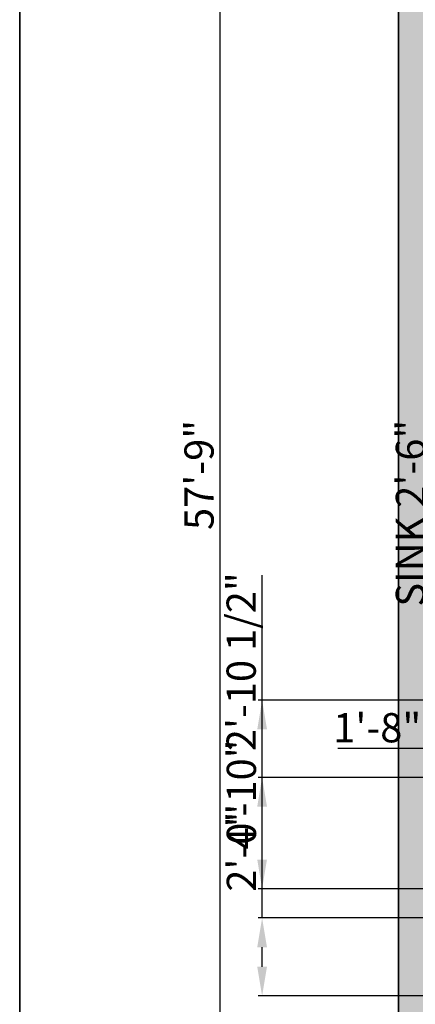
# Model space of a CAD drawing. Units: inches. Extents: x 32476 to 33108, y 58720 to 59630.
# Tile 2 of 6: x 32476 to 32598, y 58975 to 59278. Entities that reach past the tile are written whole.
import ezdxf

# ---------------------------------------------------------------- set-up
doc = ezdxf.new("R2010")
doc.units = ezdxf.units.IN
for name, color, linetype, lineweight in [('A-ANNO-DIMS', 6, 'Continuous', 18), ('A-ANNO-TTLB', 7, 'Continuous', 35), ('A-WALL', 7, 'Continuous', 35), ('A-WALL-PATT', 251, 'Continuous', 13)]:
    doc.layers.add(name, color=color, linetype=linetype, lineweight=lineweight)
doc.styles.get("Standard").update_dxf_attribs({"font": 'arial.ttf'})
doc.dimstyles.new('ISO-25', dxfattribs={"dimtxt": 9, "dimasz": 9, "dimexe": 1.25, "dimexo": 0.625, "dimtad": 1, "dimdec": 1, "dimrnd": 9, "dimlunit": 3, "dimtxsty": 'Standard', "dimcen": 2.5, "dimadec": 0, "dimazin": 0, "dimtfac": 1, "dimtdec": 1, "dimtmove": 0, "dimatfit": 3, "dimfxl": 1, "dimarcsym": 0})

# ---------------------------------------------------------------- blocks, each defined once
blk = doc.blocks.new('*D2')
at = {"layer": 'A-ANNO-DIMS', "color": 0, "lineweight": -2, "transparency": 16777216}
for p, q in [((32592.41, 59486.22), (32536.75, 59486.22)), ((32538, 59477.22), (32538, 58799.22)), ((32592.41, 58790.22), (32536.75, 58790.22))]:
    blk.add_line(p, q, dxfattribs=at)
at = {"layer": 'A-ANNO-DIMS', "color": 0, "transparency": 16777216}
for points in [[(32536.5, 59477.22), (32539.5, 59477.22), (32538, 59486.22)], [(32536.5, 58799.22), (32539.5, 58799.22), (32538, 58790.22)]]:
    blk.add_solid(points, dxfattribs=at)
at = {"layer": 'Defpoints', "color": 0, "transparency": 16777216}
for p in [(32593.04, 59486.22), (32538, 58790.22), (32593.04, 58790.22)]:
    blk.add_point(p, dxfattribs=at)
at = {"layer": 'A-ANNO-DIMS', "color": 0, "transparency": 16777216, "insert": (32532.78, 59138.22), "char_height": 9, "attachment_point": 5, "rotation": 90}
blk.add_mtext('57\'-9"', dxfattribs=at)
blk = doc.blocks.new('*D35')
at = {"layer": 'A-ANNO-DIMS', "color": 0, "lineweight": -2, "transparency": 16777216}
for p, q in [((32603.15, 59088.44), (32603.15, 59155.41)), ((32607.03, 59088.44), (32601.9, 59088.44)), ((32603.15, 59067.44), (32603.15, 59079.44)), ((32607.03, 59058.44), (32601.9, 59058.44))]:
    blk.add_line(p, q, dxfattribs=at)
at = {"layer": 'A-ANNO-DIMS', "color": 0, "transparency": 16777216}
for points in [[(32601.65, 59079.44), (32604.65, 59079.44), (32603.15, 59088.44)], [(32601.65, 59067.44), (32604.65, 59067.44), (32603.15, 59058.44)]]:
    blk.add_solid(points, dxfattribs=at)
at = {"layer": 'Defpoints', "color": 0, "transparency": 16777216}
for p in [(32603.15, 59088.44), (32607.65, 59088.44), (32607.65, 59058.44)]:
    blk.add_point(p, dxfattribs=at)
at = {"layer": 'A-ANNO-DIMS', "color": 0, "transparency": 16777216, "insert": (32597.87, 59126.43), "char_height": 9, "attachment_point": 5, "rotation": 90}
blk.add_mtext('SINK 2\'-6"', dxfattribs=at)
blk = doc.blocks.new('*D36')
at = {"layer": 'A-ANNO-DIMS', "color": 0, "lineweight": -2, "transparency": 16777216}
for p, q in [((32607.65, 59057.82), (32607.65, 59052.69)), ((32627.65, 59057.82), (32627.65, 59052.69)), ((32607.65, 59053.94), (32574.33, 59053.94)), ((32618.65, 59053.94), (32616.65, 59053.94))]:
    blk.add_line(p, q, dxfattribs=at)
at = {"layer": 'A-ANNO-DIMS', "color": 0, "transparency": 16777216}
for points in [[(32616.65, 59055.44), (32616.65, 59052.44), (32607.65, 59053.94)], [(32618.65, 59055.44), (32618.65, 59052.44), (32627.65, 59053.94)]]:
    blk.add_solid(points, dxfattribs=at)
at = {"layer": 'Defpoints', "color": 0, "transparency": 16777216}
for p in [(32607.65, 59058.44), (32627.65, 59058.44), (32607.65, 59053.94)]:
    blk.add_point(p, dxfattribs=at)
at = {"layer": 'A-ANNO-DIMS', "color": 0, "transparency": 16777216, "insert": (32586.49, 59059.16), "char_height": 9, "attachment_point": 5}
blk.add_mtext('1\'-8"', dxfattribs=at)
blk = doc.blocks.new('*D40')
at = {"layer": 'A-ANNO-DIMS', "color": 0, "lineweight": -2, "transparency": 16777216}
for p, q in [((32759.79, 59068.81), (32549.79, 59068.81)), ((32551.04, 59019.72), (32551.04, 59059.81)), ((32701.41, 59010.72), (32549.79, 59010.72))]:
    blk.add_line(p, q, dxfattribs=at)
at = {"layer": 'A-ANNO-DIMS', "color": 0, "transparency": 16777216}
for points in [[(32549.54, 59059.81), (32552.54, 59059.81), (32551.04, 59068.81)], [(32549.54, 59019.72), (32552.54, 59019.72), (32551.04, 59010.72)]]:
    blk.add_solid(points, dxfattribs=at)
at = {"layer": 'Defpoints', "color": 0, "transparency": 16777216}
for p in [(32551.04, 59068.81), (32760.42, 59068.81), (32702.04, 59010.72)]:
    blk.add_point(p, dxfattribs=at)
at = {"layer": 'A-ANNO-DIMS', "color": 0, "transparency": 16777216, "insert": (32545.82, 59039.76), "char_height": 9, "attachment_point": 5, "rotation": 90}
blk.add_mtext('4\'-10"', dxfattribs=at)
blk = doc.blocks.new('*D42')
at = {"layer": 'A-ANNO-DIMS', "color": 0, "lineweight": -2, "transparency": 16777216}
for p, q in [((32551.04, 59045.02), (32551.04, 59107.31)), ((32632.57, 59045.02), (32549.79, 59045.02)), ((32551.04, 59019.72), (32551.04, 59036.02)), ((32623.76, 59010.72), (32549.79, 59010.72))]:
    blk.add_line(p, q, dxfattribs=at)
at = {"layer": 'A-ANNO-DIMS', "color": 0, "transparency": 16777216}
for points in [[(32549.54, 59036.02), (32552.54, 59036.02), (32551.04, 59045.02)], [(32549.54, 59019.72), (32552.54, 59019.72), (32551.04, 59010.72)]]:
    blk.add_solid(points, dxfattribs=at)
at = {"layer": 'Defpoints', "color": 0, "transparency": 16777216}
for p in [(32551.04, 59045.02), (32633.2, 59045.02), (32624.39, 59010.72)]:
    blk.add_point(p, dxfattribs=at)
at = {"layer": 'A-ANNO-DIMS', "color": 0, "transparency": 16777216, "insert": (32545.76, 59080.67), "char_height": 9, "attachment_point": 5, "rotation": 90}
blk.add_mtext('2\'-10 1/2"', dxfattribs=at)
blk = doc.blocks.new('*D44')
at = {"layer": 'A-ANNO-DIMS', "color": 0, "lineweight": -2, "transparency": 16777216}
for p, q in [((32551.04, 59001.72), (32551.04, 59036.05)), ((32740.1, 59001.72), (32549.79, 59001.72)), ((32551.04, 58986.72), (32551.04, 58992.72)), ((32740.1, 58977.72), (32549.79, 58977.72))]:
    blk.add_line(p, q, dxfattribs=at)
at = {"layer": 'A-ANNO-DIMS', "color": 0, "transparency": 16777216}
for points in [[(32549.54, 58992.72), (32552.54, 58992.72), (32551.04, 59001.72)], [(32549.54, 58986.72), (32552.54, 58986.72), (32551.04, 58977.72)]]:
    blk.add_solid(points, dxfattribs=at)
at = {"layer": 'Defpoints', "color": 0, "transparency": 16777216}
for p in [(32551.04, 59001.72), (32740.73, 59001.72), (32740.73, 58977.72)]:
    blk.add_point(p, dxfattribs=at)
at = {"layer": 'A-ANNO-DIMS', "color": 0, "transparency": 16777216, "insert": (32545.82, 59023.38), "char_height": 9, "attachment_point": 5, "rotation": 90}
blk.add_mtext('2\'-0"', dxfattribs=at)

msp = doc.modelspace()

# ---------------------------------------------------------------- hatches: boundary and pattern name
at = {"layer": 'A-WALL-PATT'}
h = msp.add_hatch(color=256, dxfattribs=at)
h.dxf.hatch_style = 1
h.paths.add_polyline_path([(32602.04, 59418.72), (32606.39, 59418.72), (32606.39, 59423.22), (32602.04, 59423.22), (32602.04, 59477.22), (32698.04, 59477.22), (32698.04, 59469.73), (32702.54, 59469.73), (32702.54, 59481.72), (32867.54, 59481.72), (32867.54, 59427.72), (32860.2, 59427.72), (32860.2, 59418.72), (32867.54, 59418.72), (32935.14, 59418.72), (32935.14, 59423.22), (32872.04, 59423.22), (32872.04, 59477.22), (32968.04, 59477.22), (32968.04, 59423.22), (32962.36, 59423.22), (32962.36, 59418.72), (32968.04, 59418.72), (32968.04, 59286.72), (32867.54, 59286.72), (32832.04, 59286.72), (32828.7, 59289.44), (32818.99, 59279.82), (32823.04, 59277.72), (32823.04, 59269.52), (32832.04, 59269.52), (32832.04, 59277.72), (32867.54, 59277.72), (32968.04, 59277.72), (32968.04, 58880.22), (32925.88, 58880.22), (32925.88, 58871.22), (32968.04, 58871.22), (32968.04, 58799.22), (32823.04, 58799.22), (32823.04, 58790.22), (32977.04, 58790.22), (32977.04, 59486.22), (32867.54, 59486.22), (32702.54, 59486.22), (32593.04, 59486.22), (32593.04, 58803.66), (32602.04, 58803.66), (32602.04, 59001.72), (32624.39, 59001.72), (32624.39, 59010.72), (32602.04, 59010.72), (32602.04, 59124.72), (32648.65, 59124.72), (32648.65, 59133.72), (32602.04, 59133.72), (32602.04, 59277.72), (32757.41, 59277.72), (32757.41, 59279.22), (32742.07, 59288.84), (32739.6, 59286.72), (32702.54, 59286.72), (32602.04, 59286.72)])
h.paths.add_polyline_path([(32763.92, 59133.72), (32685.69, 59133.72), (32685.69, 59124.72), (32693.04, 59124.72), (32693.04, 59010.72), (32668.87, 59010.72), (32668.87, 59001.72), (32705.76, 59001.72), (32705.76, 59010.72), (32702.04, 59010.72), (32702.04, 59124.72), (32763.92, 59124.72)], flags=17)
h.paths.add_polyline_path([(32832.04, 59226.49), (32823.04, 59226.49), (32823.04, 59133.72), (32814.31, 59133.72), (32814.31, 59124.72), (32823.04, 59124.72), (32823.04, 59099.14), (32832.04, 59099.14), (32832.04, 59124.72), (32839.29, 59124.72), (32839.29, 59133.72), (32832.04, 59133.72)], flags=17)
h.paths.add_polyline_path([(32921.54, 59133.72), (32874.43, 59133.72), (32874.43, 59124.72), (32917.04, 59124.72), (32917.04, 59097.72), (32921.54, 59097.72), (32921.54, 59124.72)], flags=17)
h.paths.add_polyline_path([(32832.04, 59066.22), (32968.04, 59066.22), (32968.04, 59070.72), (32921.54, 59070.72), (32921.54, 59074.56), (32917.04, 59074.56), (32917.04, 59070.72), (32832.04, 59070.72), (32832.04, 59074.32), (32823.04, 59074.32), (32823.04, 59056.98), (32832.04, 59056.98)], flags=17)
h.paths.add_polyline_path([(32738.1, 59010.72), (32721.79, 59010.72), (32721.79, 59001.72), (32738.1, 59001.72)], flags=16)
h.paths.add_polyline_path([(32763.19, 59010.72), (32754.77, 59010.72), (32754.77, 59001.72), (32763.19, 59001.72)], flags=16)
h.paths.add_polyline_path([(32832.04, 59016.15), (32823.04, 59016.15), (32823.04, 59010.72), (32814.31, 59010.72), (32814.31, 59001.72), (32823.04, 59001.72), (32823.04, 58871.22), (32860.05, 58871.22), (32860.05, 58880.22), (32832.04, 58880.22)], flags=17)
h.paths.add_polyline_path([(32702.54, 59448.33), (32698.04, 59448.33), (32698.04, 59423.22), (32631.9, 59423.22), (32631.9, 59418.72), (32702.54, 59418.72), (32706.18, 59418.72), (32706.18, 59427.72), (32702.54, 59427.72)], flags=17)
h.paths.add_polyline_path([(32789.04, 59418.72), (32800.22, 59418.72), (32800.22, 59427.72), (32775.59, 59427.72), (32775.59, 59418.72), (32780.04, 59418.72), (32780.04, 59337.58), (32773.73, 59333.67), (32782.91, 59322.03), (32784.1, 59324.11), (32785.3, 59322.03), (32798.33, 59329.69), (32789.04, 59343.18)], flags=17)

# ---------------------------------------------------------------- linework, layer by layer
at = {"layer": 'A-ANNO-TTLB'}
msp.add_lwpolyline([(32476.39, 59629.64), (33046.1, 59629.64), (33046.1, 58720.03), (32476.39, 58720.03)], close=True, dxfattribs=at)
at = {"layer": 'A-WALL'}
msp.add_line((32593.04, 59486.22), (32593.04, 58790.22), dxfattribs=at)

# ---------------------------------------------------------------- dimensions: what is measured, and where the dimension line sits
at = {"layer": 'A-ANNO-DIMS'}
for base, p1, p2, angle, override, picture, middle in [((32538, 58790.22), (32593.04, 59486.22), (32593.04, 58790.22), 90, {"dimclrd": 0, "dimclre": 0, "dimclrt": 0}, '*D2', (32532.78, 59138.22)), ((32551.04, 59045.02), (32624.39, 59010.72), (32633.2, 59045.02), 90, {"dimdec": 1, "dimlfac": 1, "dimrnd": 0, "dimzin": 1, "dimdsep": 46, "dimlunit": 4, "dimfrac": 2}, '*D42', (32545.76, 59080.67)), ((32551.04, 59068.81), (32702.04, 59010.72), (32760.42, 59068.81), 90, {"dimdec": 1, "dimlfac": 1, "dimrnd": 0, "dimzin": 1, "dimdsep": 46, "dimlunit": 4, "dimfrac": 2}, '*D40', (32545.82, 59039.76)), ((32607.65, 59053.94), (32627.65, 59058.44), (32607.65, 59058.44), 180, {"dimdec": 1, "dimlfac": 1, "dimrnd": 0, "dimzin": 1, "dimdsep": 46, "dimlunit": 4, "dimfrac": 2}, '*D36', (32586.49, 59059.16)), ((32551.04, 59001.72), (32740.73, 58977.72), (32740.73, 59001.72), 90, {"dimdec": 1, "dimlfac": 1, "dimrnd": 0, "dimzin": 1, "dimdsep": 46, "dimlunit": 4, "dimfrac": 2}, '*D44', (32545.82, 59023.38))]:
    dim = msp.add_linear_dim(base=base, p1=p1, p2=p2, angle=angle, dimstyle='ISO-25', override=override, dxfattribs=at)
    dim.commit()
    dim.dimension.update_dxf_attribs({"geometry": picture, "text_midpoint": middle})
dim = msp.add_linear_dim(base=(32603.15, 59088.44), p1=(32607.65, 59058.44), p2=(32607.65, 59088.44), angle=90, text='SINK <>', dimstyle='ISO-25', override={"dimdec": 1, "dimlfac": 1, "dimrnd": 0, "dimzin": 1, "dimdsep": 46, "dimlunit": 4, "dimfrac": 2}, dxfattribs=at)
dim.commit()
dim.dimension.update_dxf_attribs({"geometry": '*D35', "text_midpoint": (32597.87, 59126.43)})

doc.saveas('drawing.dxf')
